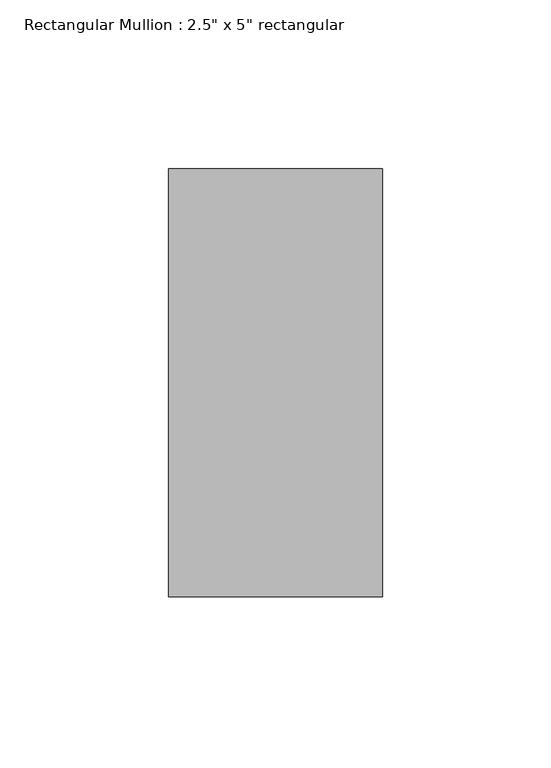
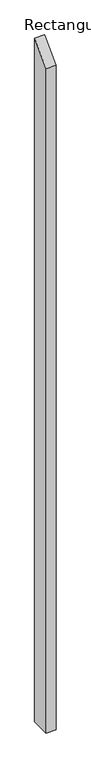
"""IFC4 building model written with IfcOpenShell, lengths in millimetres: member geometry."""

from ifc_helpers import new_model, si_unit, frame, origin, place, context, project, spatial, polyline, outline, extrude, source, transform, mapped, element, save


def member_d7cde369(model_context):
    return source(origin(), model_context, "Body", "SweptSolid", [
        extrude(outline(polyline([(-63.5, -63.5), (63.5, 63.5), (63.5, -4531.2793314), (-63.5, -4531.2793314), (-63.5, -63.5)])), frame((-63.5, 0.0, 0.0), z_axis=(1.0, 0.0, 0.0), x_axis=(0.0, 1.0, 0.0)), (0.0, 0.0, 1.0), 63.5),
    ])


if __name__ == "__main__":
    model = new_model("IFC4")
    model_context = context("Model", 3, world=origin())
    ifc_project = project(units=[si_unit("LENGTHUNIT", "METRE", prefix="MILLI")], contexts=[model_context])
    site = spatial("IfcSite", under=ifc_project)
    building = spatial("IfcBuilding", under=site)
    placement = place(None, origin())
    member_shape = member_d7cde369(model_context)
    element("IfcMember", 1, ObjectType="Rectangular Mullion : 2.5\" x 5\" rectangular", at=placement, inside=building, context=model_context, shape_type="MappedRepresentation", body=[
        mapped(member_shape, transform((0.0, 0.0, 0.0), x_axis=(1.0, 0.0, 0.0), y_axis=(0.0, 1.0, 0.0), z_axis=(0.0, 0.0, 1.0))),
    ])
    save(model, "model.ifc")

# Revit data of these elements
# Type "Rectangular Mullion : 2.5\" x 5\" rectangular"
#   built-in parameter 1007304 = 0.416667 (stored number, unit not read)
#   built-in parameter 1007301 = 0.104167 (stored number, unit not read)
#   built-in parameter 1007300 = 0.104167 (stored number, unit not read)
# Element 1 (IfcMember, "Rectangular Mullion : 2.5\" x 5\" rectangular")
#   Materials on its faces: "Aluminum"
# Materials
#   "Aluminum": class "Metal", colour RGB 247 247 247, transparency 0, Description = "Aluminum 6061", Cost = 0
